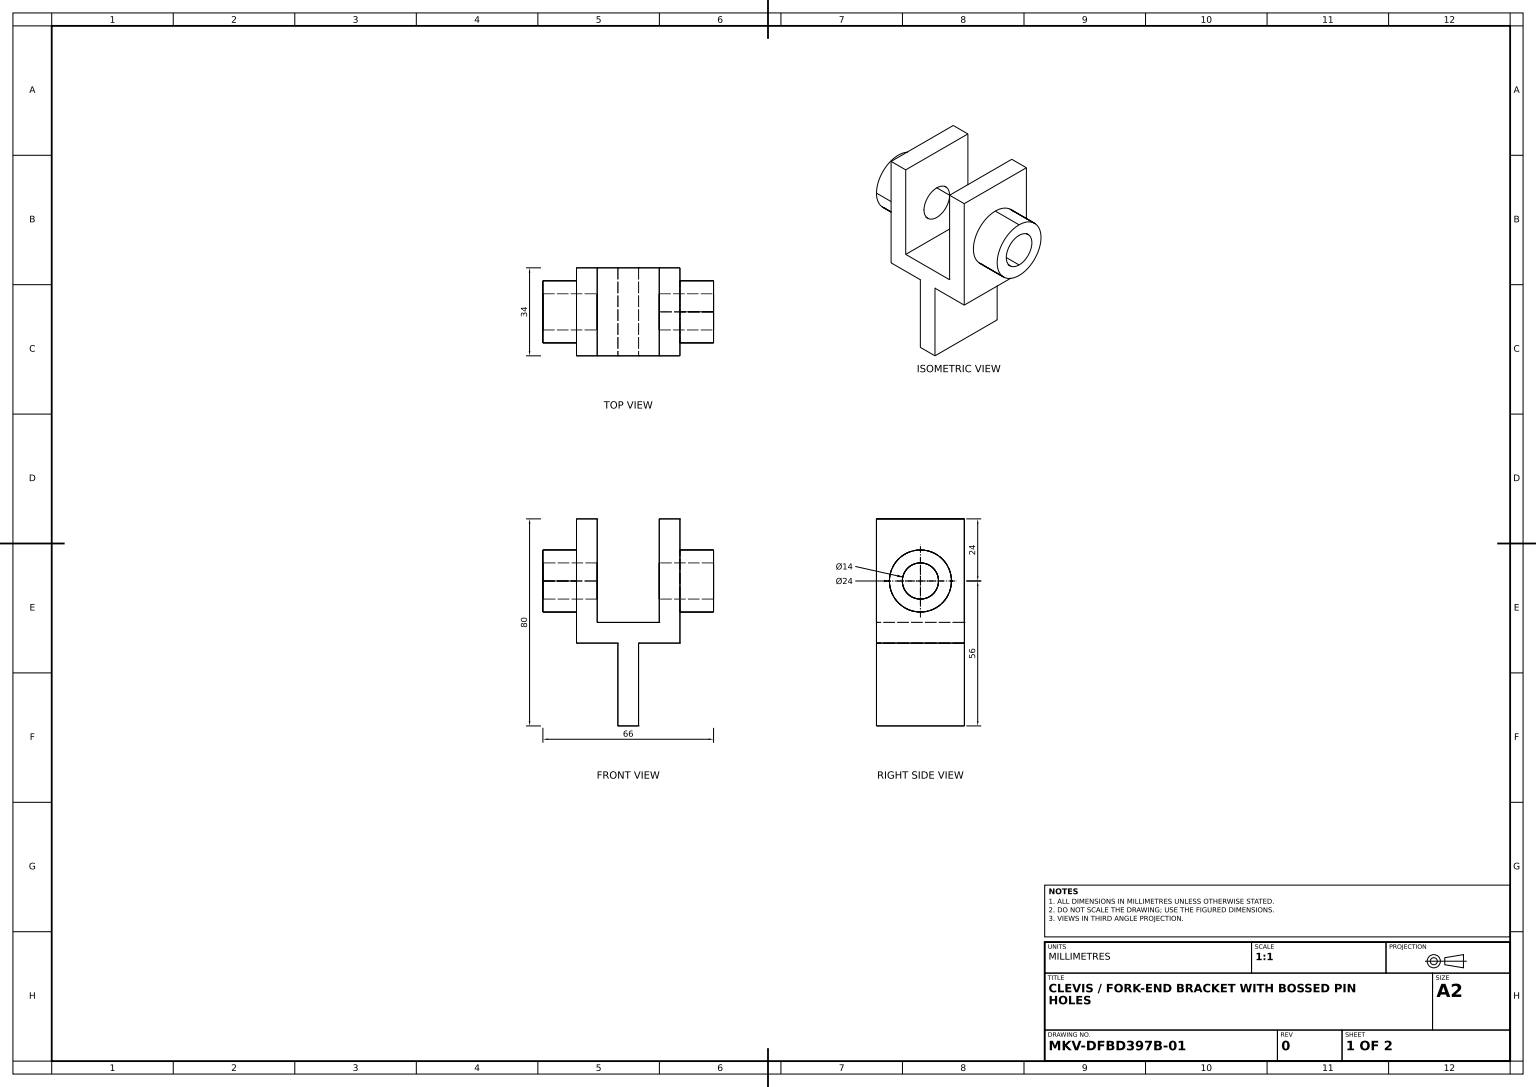
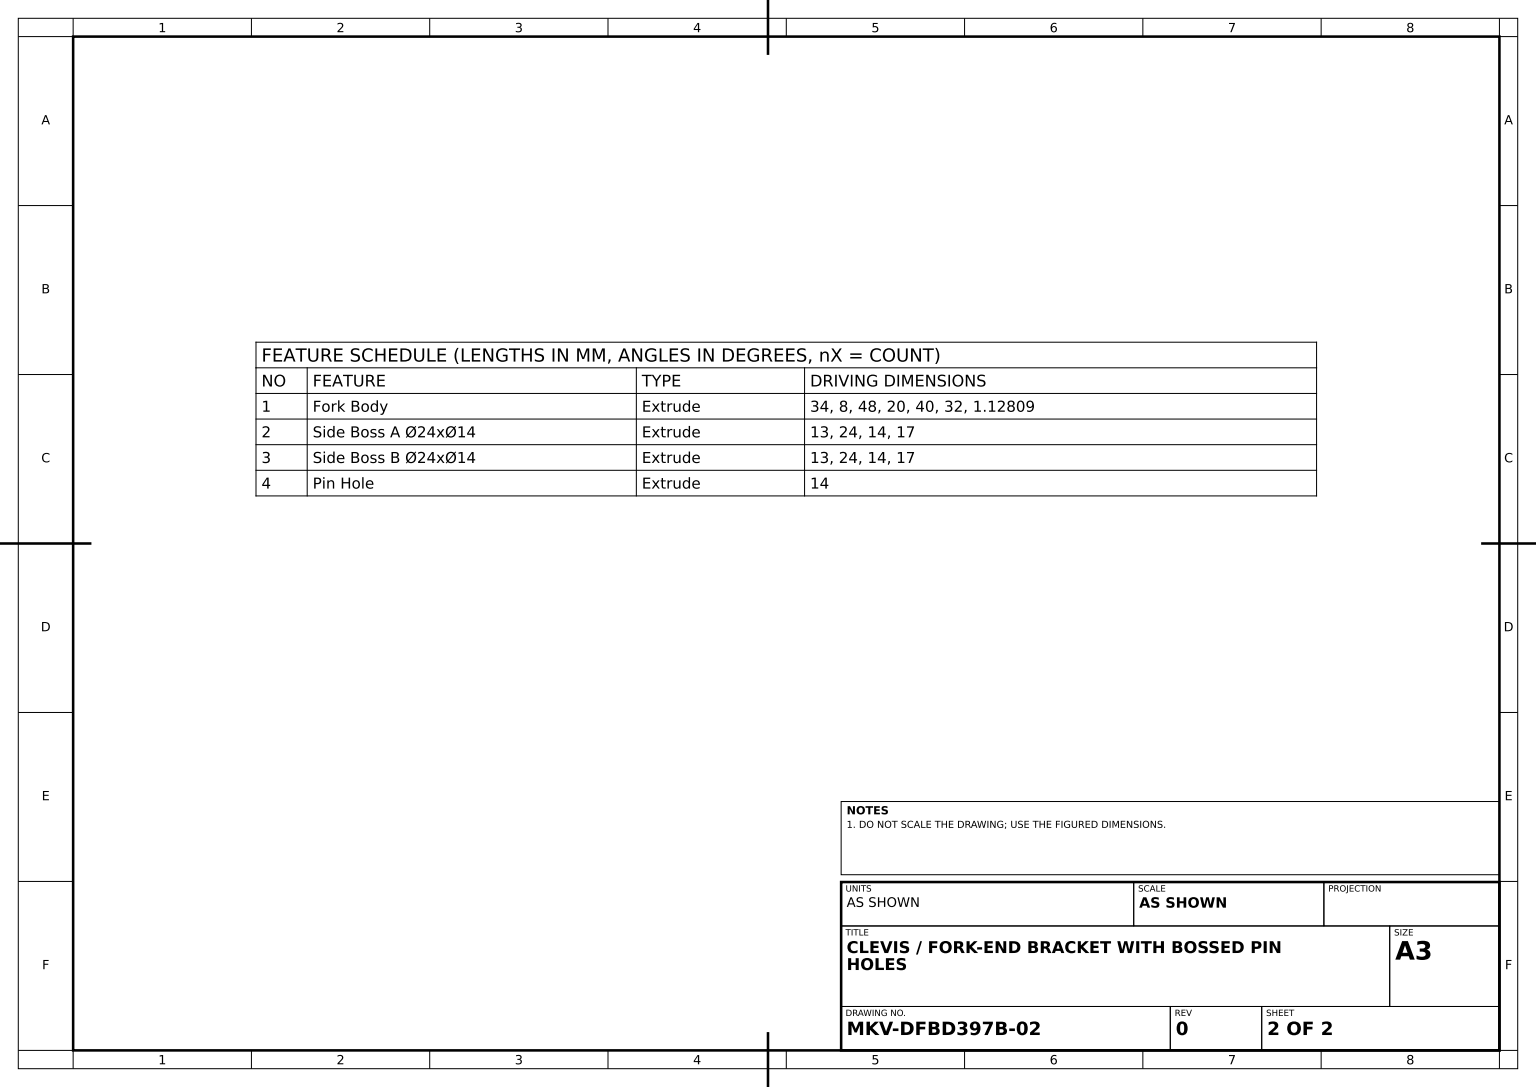
from build123d import *

# Parameters (mm, degrees)
FORK_BODY_DEPTH          = 34
SIDE_BOSS_A_SKETCH_R     = 12
SIDE_BOSS_A_SKETCH_R_2   = 7
SIDE_BOSS_A_24X_14_DEPTH = 13
SIDE_START               = 13
SIDE_BOSS_B_SKETCH_R     = 12
SIDE_BOSS_B_SKETCH_R_2   = 7
SIDE_BOSS_B_24X_14_DEPTH = 13
PIN_HOLE_SKETCH_R        = 7
PIN_HOLE_DEPTH           = 102.808644034


with BuildPart() as part:
    # Fork Profile Sketch → Fork Body (new body)
    with BuildSketch(Plane.XY):
        Polygon((-2.871912694, 0), (-2.871912694, 32), (-18.871912694, 32), (-18.871912694, 80), (-10.871912694, 80), (-10.871912694, 40), (13.128087306, 40), (13.128087306, 80), (21.128087306, 80), (21.128087306, 32), (5.128087306, 32), (5.128087306, 0), align=None)
    extrude(amount=-FORK_BODY_DEPTH)

    # Side Boss A Sketch → Side Boss A Ø24xØ14 (add)
    with BuildSketch(Plane(origin=(21.128087306, 0, 0), x_dir=(0, 0, -1), z_dir=(1, 0, 0))):
        with Locations(Location((17, 56, 0), (0, 0, 270))):
            Circle(SIDE_BOSS_A_SKETCH_R)
        with Locations(Location((17, 56, 0), (0, 0, 270))):
            Circle(SIDE_BOSS_A_SKETCH_R_2, mode=Mode.SUBTRACT)
    extrude(amount=SIDE_BOSS_A_24X_14_DEPTH)

    # Side Boss B Sketch → Side Boss B Ø24xØ14 (add)
    with BuildSketch(Plane.ZY.offset(18.871912694).offset(SIDE_START)):
        with Locations(Location((-17, 56, 0), (0, 0, 270))):
            Circle(SIDE_BOSS_B_SKETCH_R)
        with Locations(Location((-17, 56, 0), (0, 0, 270))):
            Circle(SIDE_BOSS_B_SKETCH_R_2, mode=Mode.SUBTRACT)
    extrude(amount=-SIDE_BOSS_B_24X_14_DEPTH)

    # Pin Hole Sketch → Pin Hole (cut, through all)
    with BuildSketch(Plane.ZY.offset(18.871912694)):
        with Locations(Location((-17, 56, 0), (0, 0, 270))):
            Circle(PIN_HOLE_SKETCH_R)
    extrude(amount=-PIN_HOLE_DEPTH, mode=Mode.SUBTRACT)


solid = part.part
